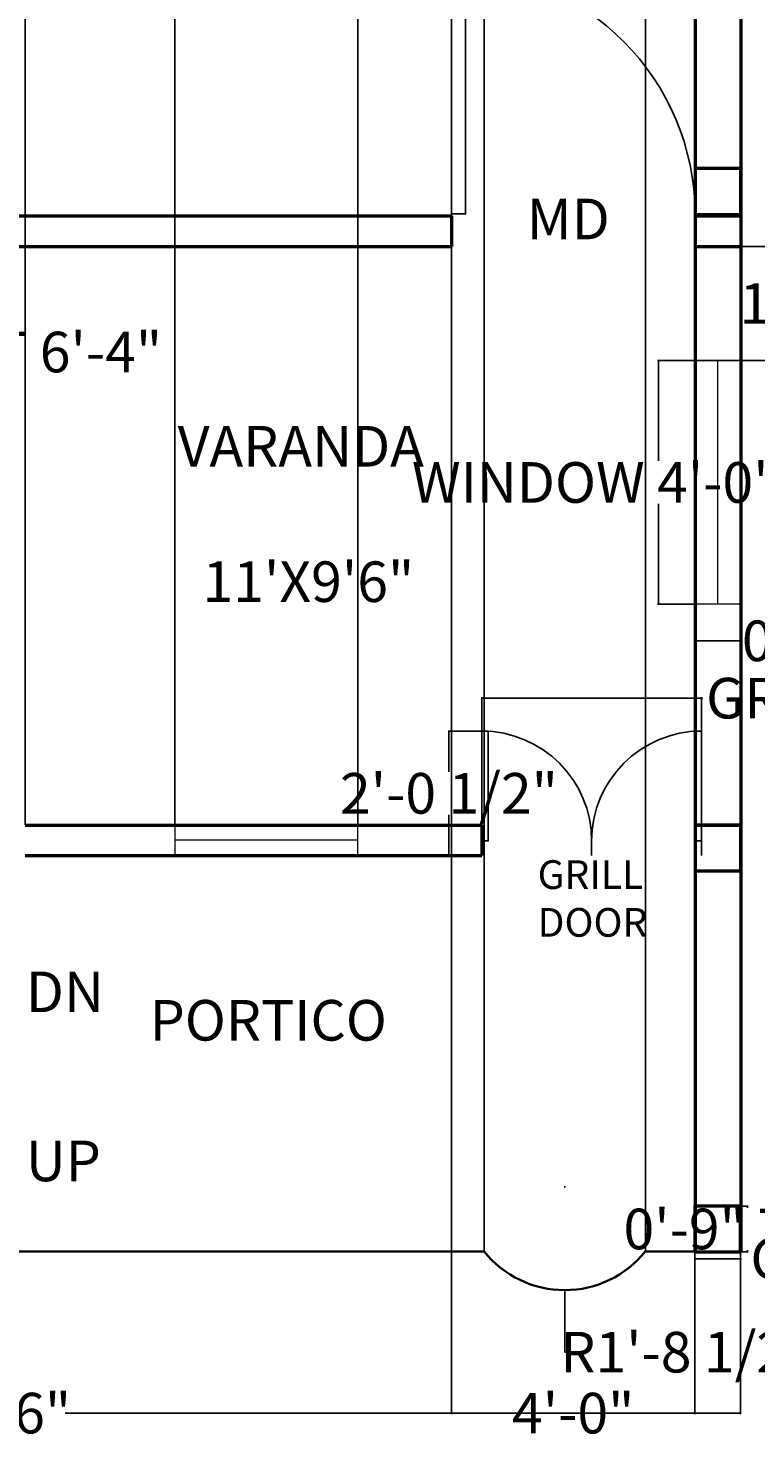
# Model space of a CAD drawing. Units: inches. Extents: x 1305 to 1889, y -508 to -5.
# Tile 6 of 8: x 1548 to 1691, y -498 to -220. Entities that reach past the tile are written whole.
import ezdxf

# ---------------------------------------------------------------- set-up
doc = ezdxf.new("R2010")
doc.units = ezdxf.units.IN
doc.header["$MEASUREMENT"] = 0
for name, color, linetype, lineweight in [('A-ANNO-DIMS', 2, 'Continuous', 18), ('A-ANNO-TEXT', 7, 'Continuous', 18), ('A-AREA-IDEN', 7, 'Continuous', 25), ('A-COLS', 7, 'Continuous', 50), ('A-DOOR', 3, 'Continuous', 25), ('A-FLOR', 7, 'Continuous', 35), ('A-GLAZ', 4, 'Continuous', 18), ('A-WALL', 7, 'Continuous', 50)]:
    doc.layers.add(name, color=color, linetype=linetype, lineweight=lineweight)
doc.styles.get("Standard").update_dxf_attribs({"font": 'arial.ttf', "height": 8})
doc.dimstyles.get("Standard").update_dxf_attribs({"dimtxt": 0.18, "dimasz": 0.18, "dimexe": 0.18, "dimexo": 0.0625, "dimgap": 0.09, "dimtad": 0, "dimtih": 1, "dimtoh": 1, "dimzin": 0, "dimdsep": 46, "dimlunit": 4, "dimtxsty": 'Standard', "dimcen": 0.09, "dimadec": 0, "dimazin": 0, "dimtfac": 1, "dimtofl": 0, "dimtmove": 0, "dimatfit": 3, "dimfxl": 1, "dimtolj": 1, "dimtzin": 0, "dimarcsym": 0})

# ---------------------------------------------------------------- blocks, each defined once
blk = doc.blocks.new('*U9')
for p, q in [((0, 0), (0, -100)), ((750, 0), (750, -100))]:
    blk.add_line(p, q)
blk.add_lwpolyline([(0, 0), (0, 750), (43.75, 750), (43.75, 0)], close=True)
blk.add_arc((0, 0), 750, 0, 90)
blk = doc.blocks.new('*U10')
for p, q in [((-750, 0), (-750, -100)), ((0, 0), (0, -100))]:
    blk.add_line(p, q)
blk.add_lwpolyline([(0, 0), (0, 750), (-43.75, 750), (-43.75, 0)], close=True)
blk.add_arc((0, 0), 750, 90, 180)
blk = doc.blocks.new('2 DOOR')
at = {"xscale": 0.0240000000000007, "yscale": 0.0240000000000007, "zscale": 0.0240000000000007}
for name, p in [('*U9', (14.89, -37.46)), ('*U10', (50.89, -37.46))]:
    blk.add_blockref(name, p, dxfattribs=at)
blk = doc.blocks.new('*U13')
for p, q in [((0, 0), (0, -100)), ((750, 0), (750, -100))]:
    blk.add_line(p, q)
blk.add_lwpolyline([(0, 0), (0, 750), (43.75, 750), (43.75, 0)], close=True)
blk.add_arc((0, 0), 750, 0, 90)
blk = doc.blocks.new('WIN-48IN')
for p, q in [((0, 9), (0, 0)), ((48, 9), (48, 0)), ((48, 4.5), (0, 4.5))]:
    blk.add_line(p, q)
blk = doc.blocks.new('COL-9X9')
blk.add_lwpolyline([(0, 0), (9, 0), (9, 9), (0, 9)], close=True)
blk = doc.blocks.new('*D30')
at = {"layer": 'A-ANNO-DIMS', "color": 0, "lineweight": -2, "transparency": 16777216}
for p, q in [((1679.05, -461.36), (1679.05, -462.83)), ((1688.05, -461.36), (1688.05, -462.83)), ((1679.23, -462.65), (1687.87, -462.65)), ((1688.05, -462.65), (1688.23, -462.65))]:
    blk.add_line(p, q, dxfattribs=at)
at = {"layer": 'A-ANNO-DIMS', "color": 0, "transparency": 16777216}
for points in [[(1679.23, -462.62), (1679.23, -462.68), (1679.05, -462.65)], [(1687.87, -462.62), (1687.87, -462.68), (1688.05, -462.65)]]:
    blk.add_solid(points, dxfattribs=at)
at = {"layer": 'Defpoints', "color": 0, "transparency": 16777216}
for p in [(1679.05, -461.3), (1688.05, -461.3), (1688.05, -462.65)]:
    blk.add_point(p, dxfattribs=at)
at = {"layer": 'A-ANNO-DIMS', "color": 0, "transparency": 16777216, "insert": (1738.43, -462.65), "char_height": 8, "attachment_point": 5}
blk.add_mtext('\\A1;COLUMN 0\'-9" TYP.', dxfattribs=at)
blk = doc.blocks.new('*D31')
at = {"layer": 'A-ANNO-DIMS', "color": 0, "lineweight": -2, "transparency": 16777216}
for p, q in [((1688.12, -452.3), (1689.58, -452.3)), ((1689.4, -452.48), (1689.4, -452.62)), ((1688.12, -461.3), (1689.58, -461.3)), ((1689.4, -461.12), (1689.4, -460.97))]:
    blk.add_line(p, q, dxfattribs=at)
at = {"layer": 'A-ANNO-DIMS', "color": 0, "transparency": 16777216}
for points in [[(1689.37, -452.48), (1689.43, -452.48), (1689.4, -452.3)], [(1689.37, -461.12), (1689.43, -461.12), (1689.4, -461.3)]]:
    blk.add_solid(points, dxfattribs=at)
at = {"layer": 'Defpoints', "color": 0, "transparency": 16777216}
for p in [(1688.05, -452.3), (1689.4, -452.3), (1688.05, -461.3)]:
    blk.add_point(p, dxfattribs=at)
at = {"layer": 'A-ANNO-DIMS', "color": 0, "transparency": 16777216, "insert": (1689.4, -456.8), "char_height": 8, "attachment_point": 5}
blk.add_mtext('\\A1;0\'-9" TYP.', dxfattribs=at)
blk = doc.blocks.new('*D32')
at = {"layer": 'A-ANNO-DIMS', "color": 0, "lineweight": -2, "transparency": 16777216}
for p, q in [((1679.01, -285.74), (1671.69, -285.74)), ((1671.87, -285.92), (1671.87, -305.51)), ((1671.87, -333.56), (1671.87, -313.97)), ((1679.01, -333.74), (1671.69, -333.74))]:
    blk.add_line(p, q, dxfattribs=at)
at = {"layer": 'A-ANNO-DIMS', "color": 0, "transparency": 16777216}
for points in [[(1671.84, -285.92), (1671.9, -285.92), (1671.87, -285.74)], [(1671.84, -333.56), (1671.9, -333.56), (1671.87, -333.74)]]:
    blk.add_solid(points, dxfattribs=at)
at = {"layer": 'Defpoints', "color": 0, "transparency": 16777216}
for p in [(1679.07, -285.74), (1671.87, -333.74), (1679.07, -333.74)]:
    blk.add_point(p, dxfattribs=at)
at = {"layer": 'A-ANNO-DIMS', "color": 0, "transparency": 16777216, "insert": (1671.87, -309.74), "char_height": 8, "attachment_point": 5}
blk.add_mtext('\\A1;WINDOW 4\'-0" TYP.', dxfattribs=at)
blk = doc.blocks.new('*D33')
at = {"layer": 'A-ANNO-DIMS', "color": 0, "lineweight": -2, "transparency": 16777216}
for p, q in [((1679.07, -333.8), (1679.07, -341.12)), ((1688.07, -333.8), (1688.07, -341.12)), ((1679.25, -340.94), (1687.89, -340.94)), ((1688.07, -340.94), (1688.25, -340.94))]:
    blk.add_line(p, q, dxfattribs=at)
at = {"layer": 'A-ANNO-DIMS', "color": 0, "transparency": 16777216}
for points in [[(1679.25, -340.91), (1679.25, -340.97), (1679.07, -340.94)], [(1687.89, -340.91), (1687.89, -340.97), (1688.07, -340.94)]]:
    blk.add_solid(points, dxfattribs=at)
at = {"layer": 'Defpoints', "color": 0, "transparency": 16777216}
for p in [(1679.07, -333.74), (1688.07, -333.74), (1688.07, -340.94)]:
    blk.add_point(p, dxfattribs=at)
at = {"layer": 'A-ANNO-DIMS', "color": 0, "transparency": 16777216, "insert": (1712.73, -340.94), "char_height": 8, "attachment_point": 5}
blk.add_mtext('\\A1;0\'-9" TYP.', dxfattribs=at)
blk = doc.blocks.new('*D40')
at = {"layer": 'A-ANNO-DIMS', "color": 0, "lineweight": -2, "transparency": 16777216}
for p, q in [((1410.93, -272.7), (1410.93, -284.23)), ((1487, -272.7), (1487, -284.23)), ((1411.11, -284.05), (1486.82, -284.05)), ((1487, -284.05), (1487.18, -284.05))]:
    blk.add_line(p, q, dxfattribs=at)
at = {"layer": 'A-ANNO-DIMS', "color": 0, "transparency": 16777216}
for points in [[(1411.11, -284.02), (1411.11, -284.08), (1410.93, -284.05)], [(1486.82, -284.02), (1486.82, -284.08), (1487, -284.05)]]:
    blk.add_solid(points, dxfattribs=at)
at = {"layer": 'Defpoints', "color": 0, "transparency": 16777216}
for p in [(1410.93, -272.64), (1487, -272.64), (1487, -284.05)]:
    blk.add_point(p, dxfattribs=at)
at = {"layer": 'A-ANNO-DIMS', "color": 0, "transparency": 16777216, "insert": (1531.23, -284.05), "char_height": 8, "attachment_point": 5}
blk.add_mtext('\\A1;DINING SET 6\'-4"', dxfattribs=at)
blk = doc.blocks.new('*D42')
at = {"layer": 'A-ANNO-DIMS', "color": 0, "lineweight": -2, "transparency": 16777216}
for p, q in [((1637.07, -358.66), (1637.07, -352.05)), ((1637.25, -352.23), (1680.16, -352.23)), ((1680.34, -358.66), (1680.34, -352.05)), ((1680.34, -352.23), (1680.52, -352.23))]:
    blk.add_line(p, q, dxfattribs=at)
at = {"layer": 'A-ANNO-DIMS', "color": 0, "transparency": 16777216}
for points in [[(1637.25, -352.2), (1637.25, -352.26), (1637.07, -352.23)], [(1680.16, -352.2), (1680.16, -352.26), (1680.34, -352.23)]]:
    blk.add_solid(points, dxfattribs=at)
at = {"layer": 'Defpoints', "color": 0, "transparency": 16777216}
for p in [(1680.34, -352.23), (1637.07, -358.72), (1680.34, -358.72)]:
    blk.add_point(p, dxfattribs=at)
at = {"layer": 'A-ANNO-DIMS', "color": 0, "transparency": 16777216, "insert": (1721.92, -352.23), "char_height": 8, "attachment_point": 5}
blk.add_mtext('\\A1;GRILLE 3\'-7 1/2"', dxfattribs=at)
blk = doc.blocks.new('*D43')
at = {"layer": 'A-ANNO-DIMS', "color": 0, "lineweight": -2, "transparency": 16777216}
for p, q in [((1637.01, -358.72), (1630.41, -358.72)), ((1630.59, -358.9), (1630.59, -366.75)), ((1630.59, -383.06), (1630.59, -375.21)), ((1637.01, -383.24), (1630.41, -383.24))]:
    blk.add_line(p, q, dxfattribs=at)
at = {"layer": 'A-ANNO-DIMS', "color": 0, "transparency": 16777216}
for points in [[(1630.56, -358.9), (1630.62, -358.9), (1630.59, -358.72)], [(1630.56, -383.06), (1630.62, -383.06), (1630.59, -383.24)]]:
    blk.add_solid(points, dxfattribs=at)
at = {"layer": 'Defpoints', "color": 0, "transparency": 16777216}
for p in [(1630.59, -358.72), (1637.07, -358.72), (1637.07, -383.24)]:
    blk.add_point(p, dxfattribs=at)
at = {"layer": 'A-ANNO-DIMS', "color": 0, "transparency": 16777216, "insert": (1630.59, -370.98), "char_height": 8, "attachment_point": 5}
blk.add_mtext('\\A1;2\'-0 1/2"', dxfattribs=at)
blk = doc.blocks.new('*D50')
at = {"layer": 'A-ANNO-DIMS', "color": 0, "lineweight": -2, "transparency": 16777216}
for p, q in [((1394.07, -461.3), (1394.07, -493.26)), ((1688.05, -461.36), (1688.05, -493.26)), ((1394.25, -493.08), (1527.16, -493.08)), ((1687.87, -493.08), (1554.96, -493.08))]:
    blk.add_line(p, q, dxfattribs=at)
at = {"layer": 'A-ANNO-DIMS', "color": 0, "transparency": 16777216}
for points in [[(1394.25, -493.05), (1394.25, -493.11), (1394.07, -493.08)], [(1687.87, -493.05), (1687.87, -493.11), (1688.05, -493.08)]]:
    blk.add_solid(points, dxfattribs=at)
at = {"layer": 'Defpoints', "color": 0, "transparency": 16777216}
for p in [(1394.07, -461.24), (1688.05, -461.3), (1688.05, -493.08)]:
    blk.add_point(p, dxfattribs=at)
at = {"layer": 'A-ANNO-DIMS', "color": 0, "transparency": 16777216, "insert": (1541.06, -493.08), "char_height": 8, "attachment_point": 5}
blk.add_mtext('\\A1;24\'-6"', dxfattribs=at)
blk = doc.blocks.new('*D60')
at = {"layer": 'A-ANNO-DIMS', "color": 0, "lineweight": -2, "transparency": 16777216}
for p, q in [((1631.07, -263.3), (1631.07, -493.26)), ((1679.07, -263.3), (1679.07, -493.26)), ((1631.25, -493.08), (1644.19, -493.08)), ((1678.89, -493.08), (1665.96, -493.08))]:
    blk.add_line(p, q, dxfattribs=at)
at = {"layer": 'A-ANNO-DIMS', "color": 0, "transparency": 16777216}
for points in [[(1631.25, -493.05), (1631.25, -493.11), (1631.07, -493.08)], [(1678.89, -493.05), (1678.89, -493.11), (1679.07, -493.08)]]:
    blk.add_solid(points, dxfattribs=at)
at = {"layer": 'Defpoints', "color": 0, "transparency": 16777216}
for p in [(1631.07, -263.24), (1679.07, -263.24), (1679.07, -493.08)]:
    blk.add_point(p, dxfattribs=at)
at = {"layer": 'A-ANNO-DIMS', "color": 0, "transparency": 16777216, "insert": (1655.07, -493.08), "char_height": 8, "attachment_point": 5}
blk.add_mtext('\\A1;4\'-0"', dxfattribs=at)
blk = doc.blocks.new('*D63')
at = {"layer": 'A-ANNO-DIMS', "color": 0, "lineweight": -2, "transparency": 16777216}
for p, q in [((1637.53, -461.18), (1637.53, -85.83)), ((1637.71, -86.01), (1642.61, -86.01)), ((1669.11, -86.01), (1664.2, -86.01)), ((1669.29, -461.18), (1669.29, -85.83))]:
    blk.add_line(p, q, dxfattribs=at)
at = {"layer": 'A-ANNO-DIMS', "color": 0, "transparency": 16777216}
for points in [[(1637.71, -85.98), (1637.71, -86.04), (1637.53, -86.01)], [(1669.11, -85.98), (1669.11, -86.04), (1669.29, -86.01)]]:
    blk.add_solid(points, dxfattribs=at)
at = {"layer": 'Defpoints', "color": 0, "transparency": 16777216}
for p in [(1669.29, -86.01), (1637.53, -461.24), (1669.29, -461.24)]:
    blk.add_point(p, dxfattribs=at)
at = {"layer": 'A-ANNO-DIMS', "color": 0, "transparency": 16777216, "insert": (1653.41, -86.01), "char_height": 8, "attachment_point": 5}
blk.add_mtext('\\A1;2\'-8"', dxfattribs=at)
blk = doc.blocks.new('*D64')
at = {"layer": 'A-ANNO-DIMS', "color": 0, "lineweight": -2, "transparency": 16777216}
for p, q in [((1669.29, -461.18), (1669.29, -85.83)), ((1669.47, -86.01), (1687.87, -86.01)), ((1688.05, -461.23), (1688.05, -85.83)), ((1688.05, -86.01), (1688.23, -86.01))]:
    blk.add_line(p, q, dxfattribs=at)
at = {"layer": 'A-ANNO-DIMS', "color": 0, "transparency": 16777216}
for points in [[(1669.47, -85.98), (1669.47, -86.04), (1669.29, -86.01)], [(1687.87, -85.98), (1687.87, -86.04), (1688.05, -86.01)]]:
    blk.add_solid(points, dxfattribs=at)
at = {"layer": 'Defpoints', "color": 0, "transparency": 16777216}
for p in [(1688.05, -86.01), (1669.29, -461.24), (1688.05, -461.3)]:
    blk.add_point(p, dxfattribs=at)
at = {"layer": 'A-ANNO-DIMS', "color": 0, "transparency": 16777216, "insert": (1698.58, -86.01), "char_height": 8, "attachment_point": 5}
blk.add_mtext('\\A1;1\'-7"', dxfattribs=at)
blk = doc.blocks.new('*D68')
at = {"layer": 'A-ANNO-DIMS', "color": 0, "lineweight": -2, "transparency": 16777216}
for p, q in [((1679.14, -263.24), (1712.53, -263.24)), ((1712.35, -263.42), (1712.35, -270.26)), ((1712.35, -285.56), (1712.35, -278.71)), ((1679.14, -285.74), (1712.53, -285.74))]:
    blk.add_line(p, q, dxfattribs=at)
at = {"layer": 'A-ANNO-DIMS', "color": 0, "transparency": 16777216}
for points in [[(1712.32, -263.42), (1712.38, -263.42), (1712.35, -263.24)], [(1712.32, -285.56), (1712.38, -285.56), (1712.35, -285.74)]]:
    blk.add_solid(points, dxfattribs=at)
at = {"layer": 'Defpoints', "color": 0, "transparency": 16777216}
for p in [(1679.07, -263.24), (1679.07, -285.74), (1712.35, -285.74)]:
    blk.add_point(p, dxfattribs=at)
at = {"layer": 'A-ANNO-DIMS', "color": 0, "transparency": 16777216, "insert": (1712.35, -274.49), "char_height": 8, "attachment_point": 5}
blk.add_mtext('\\A1;1\'-10 1/2"', dxfattribs=at)
blk = doc.blocks.new('*D69')
at = {"layer": 'A-ANNO-DIMS', "color": 0, "lineweight": -2, "transparency": 16777216}
for p, q in [((1547.07, -377.18), (1547.07, -85.83)), ((1547.25, -86.01), (1576.42, -86.01)), ((1576.6, -377.18), (1576.6, -85.83)), ((1576.6, -86.01), (1576.78, -86.01))]:
    blk.add_line(p, q, dxfattribs=at)
at = {"layer": 'A-ANNO-DIMS', "color": 0, "transparency": 16777216}
for points in [[(1547.25, -85.98), (1547.25, -86.04), (1547.07, -86.01)], [(1576.42, -85.98), (1576.42, -86.04), (1576.6, -86.01)]]:
    blk.add_solid(points, dxfattribs=at)
at = {"layer": 'Defpoints', "color": 0, "transparency": 16777216}
for p in [(1576.6, -86.01), (1547.07, -377.24), (1576.6, -377.24)]:
    blk.add_point(p, dxfattribs=at)
at = {"layer": 'A-ANNO-DIMS', "color": 0, "transparency": 16777216, "insert": (1596.89, -86.01), "char_height": 8, "attachment_point": 5}
blk.add_mtext('\\A1;2\'-5 1/2"', dxfattribs=at)
blk = doc.blocks.new('*D70')
at = {"layer": 'A-ANNO-DIMS', "color": 0, "lineweight": -2, "transparency": 16777216}
for p, q in [((1576.6, -377.18), (1576.6, -85.83)), ((1576.78, -86.01), (1583.88, -86.01)), ((1612.42, -86.01), (1605.32, -86.01)), ((1612.6, -377.18), (1612.6, -85.83))]:
    blk.add_line(p, q, dxfattribs=at)
at = {"layer": 'A-ANNO-DIMS', "color": 0, "transparency": 16777216}
for points in [[(1576.78, -85.98), (1576.78, -86.04), (1576.6, -86.01)], [(1612.42, -85.98), (1612.42, -86.04), (1612.6, -86.01)]]:
    blk.add_solid(points, dxfattribs=at)
at = {"layer": 'Defpoints', "color": 0, "transparency": 16777216}
for p in [(1612.6, -86.01), (1576.6, -377.24), (1612.6, -377.24)]:
    blk.add_point(p, dxfattribs=at)
at = {"layer": 'A-ANNO-DIMS', "color": 0, "transparency": 16777216, "insert": (1594.6, -86.01), "char_height": 8, "attachment_point": 5}
blk.add_mtext('\\A1;3\'-0"', dxfattribs=at)
blk = doc.blocks.new('*D74')
at = {"layer": 'A-ANNO-DIMS', "color": 0, "lineweight": -2, "transparency": 16777216}
for p, q in [((1653.32, -448.48), (1653.5, -448.48)), ((1653.41, -448.57), (1653.41, -448.39)), ((1653.41, -481.07), (1653.41, -469.03)), ((1653.59, -481.07), (1653.41, -481.07))]:
    blk.add_line(p, q, dxfattribs=at)
at = {"layer": 'A-ANNO-DIMS', "color": 0, "transparency": 16777216}
blk.add_solid([(1653.44, -469.03), (1653.38, -469.03), (1653.41, -468.85)], dxfattribs=at)
at = {"layer": 'Defpoints', "color": 0, "transparency": 16777216}
for p in [(1653.41, -448.48), (1653.41, -468.85)]:
    blk.add_point(p, dxfattribs=at)
at = {"layer": 'A-ANNO-DIMS', "color": 0, "transparency": 16777216, "insert": (1677.46, -481.07), "char_height": 8, "attachment_point": 5}
blk.add_mtext('\\A1;R1\'-8 1/2"', dxfattribs=at)

msp = doc.modelspace()

# ---------------------------------------------------------------- linework, layer by layer
at = {"layer": 'A-FLOR'}
for p, q in [((1394.074, -461.239), (1637.526, -461.239)), ((1669.285, -461.239), (1688.074, -461.239))]:
    msp.add_line(p, q, dxfattribs=at)
msp.add_arc((1653.406, -448.483), 20.368, 218.77487, 321.22513, dxfattribs=at)
at = {"layer": 'A-GLAZ'}
for p, q in [((1576.598, -377.239), (1576.598, -383.239)), ((1612.598, -377.239), (1612.598, -383.239)), ((1612.598, -380.239), (1576.598, -380.239))]:
    msp.add_line(p, q, dxfattribs=at)
at = {"layer": 'A-WALL'}
for p, q in [((1679.074, -110.239), (1679.074, -461.239)), ((1688.074, -110.239), (1688.074, -461.239)), ((1541.074, -257.239), (1631.074, -257.239)), ((1631.074, -257.239), (1631.074, -263.239)), ((1679.074, -257.239), (1688.074, -257.239)), ((1541.074, -263.239), (1631.074, -263.239)), ((1679.074, -263.239), (1688.074, -263.239)), ((1547.074, -377.239), (1637.074, -377.239)), ((1637.074, -377.239), (1637.074, -383.239)), ((1679.074, -377.239), (1688.074, -377.239)), ((1547.074, -383.239), (1637.074, -383.239)), ((1679.074, -383.239), (1679.084, -383.239)), ((1688.074, -383.239), (1688.084, -383.239))]:
    msp.add_line(p, q, dxfattribs=at)

# ---------------------------------------------------------------- block references
at = {"layer": 'A-COLS'}
for p in [(1679.128, -256.923), (1679.084, -386.222), (1679.054, -461.295)]:
    msp.add_blockref('COL-9X9', p, dxfattribs=at)
at = {"layer": 'A-DOOR'}
for name, p, xscale, yscale, zscale in [('*U13', (1631.074, -256.839), 0.0640000000000004, 0.0640000000000004, 0.0640000000000004), ('2 DOOR', (1619.177, -335.336), 1.201716738197423, 1.201716738197423, 1.201716738197423)]:
    msp.add_blockref(name, p, dxfattribs=dict(at, xscale=xscale, yscale=yscale, zscale=zscale))
at = {"layer": 'A-GLAZ', "rotation": 269.9999999999999}
msp.add_blockref('WIN-48IN', (1679.074, -285.739), dxfattribs=at)

# ---------------------------------------------------------------- texts
at = {"layer": 'A-ANNO-TEXT', "attachment_point": 1}
for s, width, gutter_width, insert, char_height in [('MD', 13.3749, 40, (1645.908, -253.846), 8), ('GRILL DOOR', 14.68095, 28.228, (1648.061, -384.166), 5.6457), ('DN', 11.32348, 40, (1547.208, -406.088), 8), ('UP', 11.32348, 40, (1547.208, -439.39), 8)]:
    msp.add_mtext_dynamic_manual_height_columns(s, width=width, gutter_width=gutter_width, heights=[0], dxfattribs=dict(at, insert=insert, char_height=char_height))
at = {"layer": 'A-AREA-IDEN', "char_height": 8, "attachment_point": 1}
for s, insert in [('VARANDA\\P\\P  11\'X9\'6"', (1577.136, -298.621)), ('PORTICO', (1571.625, -411.693))]:
    msp.add_mtext_dynamic_manual_height_columns(s, width=69.27903, gutter_width=40, heights=[0], dxfattribs=dict(at, insert=insert))

# ---------------------------------------------------------------- dimensions: what is measured, and where the dimension line sits
at = {"layer": 'A-ANNO-DIMS'}
for base, p1, p2, picture, middle in [((1576.598, -86.014), (1547.074, -377.239), (1576.598, -377.239), '*D69', (1596.889, -86.014)), ((1612.598, -86.014), (1576.598, -377.239), (1612.598, -377.239), '*D70', (1594.598, -86.014)), ((1669.285, -86.014), (1637.526, -461.239), (1669.285, -461.239), '*D63', (1653.406, -86.014)), ((1688.053, -86.014), (1669.285, -461.239), (1688.053, -461.295), '*D64', (1698.58, -86.014)), ((1679.074, -493.076), (1631.074, -263.239), (1679.074, -263.239), '*D60', (1655.074, -493.076)), ((1688.053, -493.076), (1394.074, -461.239), (1688.053, -461.295), '*D50', (1541.064, -493.076))]:
    dim = msp.add_linear_dim(base=base, p1=p1, p2=p2, dimstyle='Standard', override={"dimdec": 1, "dimlfac": 1, "dimrnd": 0, "dimzin": 1, "dimdsep": 46, "dimlunit": 4, "dimfrac": 2}, dxfattribs=at)
    dim.commit()
    dim.dimension.update_dxf_attribs({"geometry": picture, "text_midpoint": middle})
for base, p1, p2, picture, middle in [((1712.353, -285.739), (1679.074, -263.239), (1679.074, -285.739), '*D68', (1712.353, -274.489)), ((1630.585, -358.723), (1637.074, -383.239), (1637.074, -358.723), '*D43', (1630.585, -370.981))]:
    dim = msp.add_linear_dim(base=base, p1=p1, p2=p2, angle=90, dimstyle='Standard', override={"dimdec": 1, "dimlfac": 1, "dimrnd": 0, "dimzin": 1, "dimdsep": 46, "dimlunit": 4, "dimfrac": 2}, dxfattribs=at)
    dim.commit()
    dim.dimension.update_dxf_attribs({"geometry": picture, "text_midpoint": middle})
for base, p1, p2, text, picture, middle in [((1487, -284.052), (1410.934, -272.642), (1487, -272.642), 'DINING SET <>', '*D40', (1531.234, -284.052)), ((1688.074, -340.939), (1679.074, -333.739), (1688.074, -333.739), '<> TYP.', '*D33', (1712.726, -340.939)), ((1680.336, -352.234), (1637.074, -358.723), (1680.336, -358.723), 'GRILLE <>', '*D42', (1721.924, -352.234)), ((1688.053, -462.645), (1679.053, -461.295), (1688.053, -461.295), 'COLUMN <> TYP.', '*D30', (1738.427, -462.645))]:
    dim = msp.add_linear_dim(base=base, p1=p1, p2=p2, text=text, dimstyle='Standard', override={"dimdec": 1, "dimlfac": 1, "dimrnd": 0, "dimzin": 1, "dimdsep": 46, "dimlunit": 4, "dimfrac": 2}, dxfattribs=at)
    dim.commit()
    dim.dimension.update_dxf_attribs({"geometry": picture, "text_midpoint": middle})
for base, p1, p2, angle, text, picture, middle in [((1671.874, -333.739), (1679.074, -285.739), (1679.074, -333.739), 270, 'WINDOW <> TYP.', '*D32', (1671.874, -309.739)), ((1689.403, -452.295), (1688.053, -461.295), (1688.053, -452.295), 90, '<> TYP.', '*D31', (1689.403, -456.795))]:
    dim = msp.add_linear_dim(base=base, p1=p1, p2=p2, angle=angle, text=text, dimstyle='Standard', override={"dimdec": 1, "dimlfac": 1, "dimrnd": 0, "dimzin": 1, "dimdsep": 46, "dimlunit": 4, "dimfrac": 2}, dxfattribs=at)
    dim.commit()
    dim.dimension.update_dxf_attribs({"geometry": picture, "text_midpoint": middle})
dim = msp.add_radius_dim(center=(1653.406, -448.483), mpoint=(1653.406, -468.851), dimstyle='Standard', override={"dimdec": 1, "dimlfac": 1, "dimrnd": 0, "dimzin": 1, "dimdsep": 46, "dimlunit": 4, "dimfrac": 2}, dxfattribs=at)
dim.commit()
dim.dimension.update_dxf_attribs({"geometry": '*D74', "text_midpoint": (1677.458, -481.072), "dimtype": 164})

doc.saveas('drawing.dxf')
